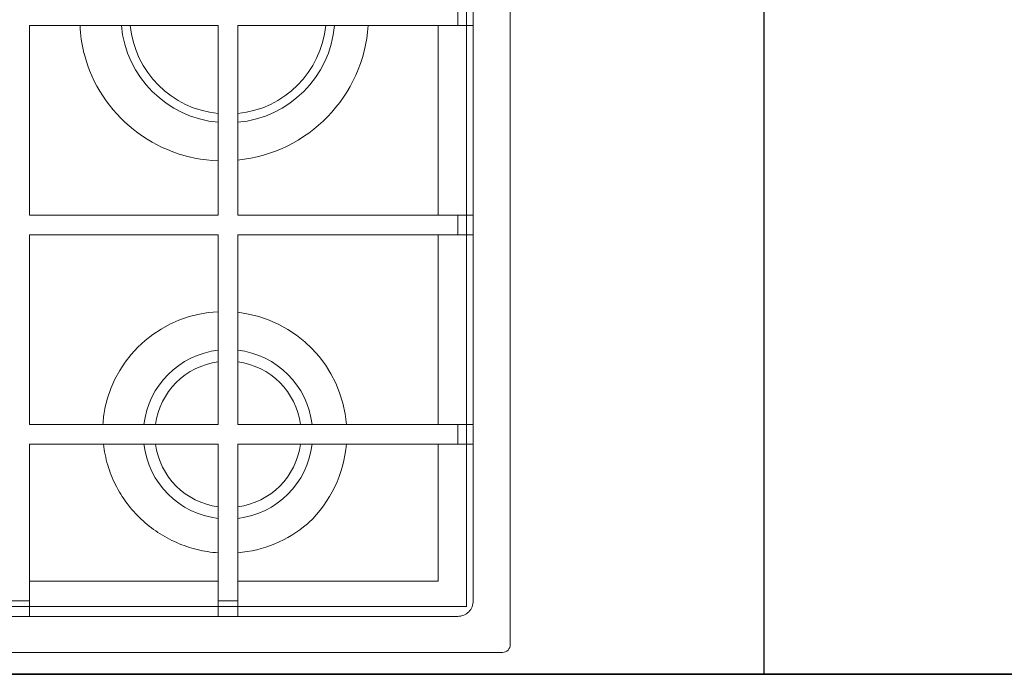
# Model space of a CAD drawing. Units: inches. Extents: x -1198 to -69, y -512 to 437.
# Tile 8 of 50: x -956 to -934, y 161 to 176. Entities that reach past the tile are written whole.
import ezdxf

# ---------------------------------------------------------------- set-up
doc = ezdxf.new("R2010")
doc.units = ezdxf.units.IN
doc.header["$MEASUREMENT"] = 0
for name, color, linetype, lineweight in [('0_Pen_No__7', 7, 'Continuous', 18), ('A-EQPM', 60, 'Continuous', 18), ('A-FLOR-CASE', 7, 'Continuous', 25), ('A-WALL', 7, 'Continuous', 35)]:
    doc.layers.add(name, color=color, linetype=linetype, lineweight=lineweight)

# ---------------------------------------------------------------- blocks, each defined once
blk = doc.blocks.new('new block')
at = {"layer": '0_Pen_No__7'}
for p, q in [((-201.32, 567.06), (-190.06, 567.06)), ((-80.82, 567.06), (-69.55, 567.06)), ((-190.06, 555.8), (-80.82, 555.8)), ((-328.59, 465.14), (-328.59, 476.4)), ((-317.33, 355.33), (-317.33, 465.14)), ((-328.59, 344.07), (-328.59, 355.33)), ((-317.33, 344.07), (-317.33, 234.26)), ((-328.59, 234.26), (-328.59, 223))]:
    blk.add_line(p, q, dxfattribs=at)
for points in [[(-354.49, 596.91), (481.18, 596.91, -0.414214), (485.68, 592.4), (485.68, 99.11), (486.24, 99.11), (486.24, 95.73), (485.68, 95.73), (485.68, 4.5, -0.414214), (481.18, 0), (-354.49, 0, -0.414214), (-359, 4.5), (-359, 95.73), (-359.56, 95.73), (-359.56, 99.11), (-359, 99.11), (-359, 592.4, -0.414214)], [(464.28, 132.33), (464.28, 567.06, 0.414214), (455.27, 576.07), (-328.59, 576.07, 0.414214), (-337.6, 567.06), (-337.6, 132.33, 0.414214), (-328.59, 123.32), (455.27, 123.32, 0.414214)]]:
    blk.add_lwpolyline(points, format="xyb", close=True, dxfattribs=at)
for points in [[(-201.32, 576.07), (-201.32, 476.4), (-337.6, 476.4)], [(-80.82, 576.07), (-80.82, 476.4), (-190.06, 476.4), (-190.06, 576.07)], [(-317.33, 476.4), (-317.33, 555.8), (-201.32, 555.8)], [(-123.65, 476.4), (-123.84, 477.94), (-124.06, 479.47), (-124.32, 481), (-124.61, 482.53), (-124.94, 484.04), (-125.29, 485.55), (-125.69, 487.05), (-126.11, 488.55), (-126.57, 490.03), (-127.06, 491.5), (-127.58, 492.96), (-128.14, 494.41), (-128.73, 495.84), (-129.35, 497.26), (-130, 498.67), (-130.68, 500.06), (-131.4, 501.44), (-132.14, 502.8), (-132.91, 504.15), (-133.71, 505.47), (-134.55, 506.78), (-135.4, 508.08), (-136.29, 509.35), (-137.21, 510.6), (-138.15, 511.83), (-139.12, 513.04), (-140.11, 514.23), (-141.14, 515.4), (-142.18, 516.54), (-143.25, 517.67), (-144.35, 518.76), (-145.46, 519.84), (-146.61, 520.89), (-147.77, 521.92), (-148.95, 522.92), (-150.16, 523.89), (-151.39, 524.84), (-152.63, 525.76), (-153.9, 526.66), (-155.19, 527.52), (-156.49, 528.36), (-157.81, 529.18), (-159.15, 529.96), (-160.51, 530.71), (-161.88, 531.44), (-163.26, 532.14), (-164.66, 532.8), (-166.08, 533.44), (-167.51, 534.05), (-168.95, 534.62), (-170.4, 535.17), (-171.86, 535.68), (-173.34, 536.16), (-174.82, 536.62), (-176.31, 537.04), (-177.82, 537.42), (-179.33, 537.78), (-180.85, 538.1), (-182.37, 538.4), (-183.9, 538.65), (-185.43, 538.88), (-186.97, 539.07), (-188.52, 539.23), (-190.06, 539.36)], [(-337.6, 465.14), (-201.32, 465.14), (-201.32, 355.33), (-337.6, 355.33)], [(-337.6, 234.26), (-201.32, 234.26), (-201.32, 344.07), (-337.6, 344.07)]]:
    blk.add_lwpolyline(points, dxfattribs=at)
for points in [[(-333.7, 12.95), (460.3, 12.95), (460.3, 570.44), (-333.7, 570.44)], [(-190.06, 355.33), (-190.06, 465.14), (-80.82, 465.14), (-80.82, 355.33)], [(-80.82, 234.26), (-80.82, 344.07), (-190.06, 344.07), (-190.06, 234.26)]]:
    blk.add_lwpolyline(points, close=True, dxfattribs=at)
for centre, radius, start, end in [((-195.46, 468.12), 71.42, 94.7107, 130.2725), ((-193.79, 470.71), 70.6, 133.5531, 175.3792), ((-195.69, 470.77), 48.99, 96.6007, 173.3993), ((-228.93, 507.66), 19.61, 130.342, 133.5279), ((-195.69, 470.77), 48.99, 6.6007, 83.3993), ((-195.69, 470.77), 42.35, 97.6426, 172.3569), ((-195.69, 470.77), 42.35, 7.6431, 82.3574), ((-193.46, 470.72), 70.94, 184.5179, 263.6357), ((-195.69, 470.77), 48.99, 186.6007, 263.3993), ((-195.69, 470.77), 42.35, 187.6431, 262.3574), ((-195.69, 470.77), 48.99, 276.6007, 353.3993), ((-195.69, 470.77), 42.35, 277.6426, 352.3569), ((-192.72, 468.81), 69.49, 349.3925, 356.9689), ((-142.89, 459.48), 18.78, 348.1147, 349.3923), ((-193.31, 470.1), 70.32, 272.6475, 348.1039), ((-193.03, 228.66), 83.93, 95.6702, 176.1745), ((-192.8, 229.51), 83.08, 14.6793, 88.1082), ((-195.69, 228.63), 61.94, 95.2168, 174.7836), ((-195.69, 228.63), 56.88, 95.6822, 174.3178), ((-195.69, 228.63), 61.94, 5.2164, 84.7832), ((-195.69, 228.63), 56.88, 5.6822, 84.3178), ((-130.93, 245.73), 19.12, 13.6505, 14.6398), ((-191.8, 230.95), 81.75, 2.3165, 13.6452)]:
    blk.add_arc(centre, radius, start, end, dxfattribs=at)
blk = doc.blocks.new('COUNTER-L')
at = {"ltscale": 10}
blk.add_line((49.349, 0), (49.349, 24), dxfattribs=at)

msp = doc.modelspace()

# ---------------------------------------------------------------- linework, layer by layer
at = {"layer": 'A-WALL', "ltscale": 10}
msp.add_line((-886.7509, 161.2277), (-1012.7509, 161.2277), dxfattribs=at)

# ---------------------------------------------------------------- block references
at = {"layer": 'A-EQPM', "xscale": 0.0393700787401575, "yscale": 0.0393700787401575, "zscale": 0.0393700787401575, "rotation": 180}
msp.add_blockref('new block', (-959.3186, 185.2277), dxfattribs=at)
at = {"layer": 'A-FLOR-CASE'}
msp.add_blockref('COUNTER-L', (-988.751, 161.228), dxfattribs=at)

doc.saveas('drawing.dxf')
